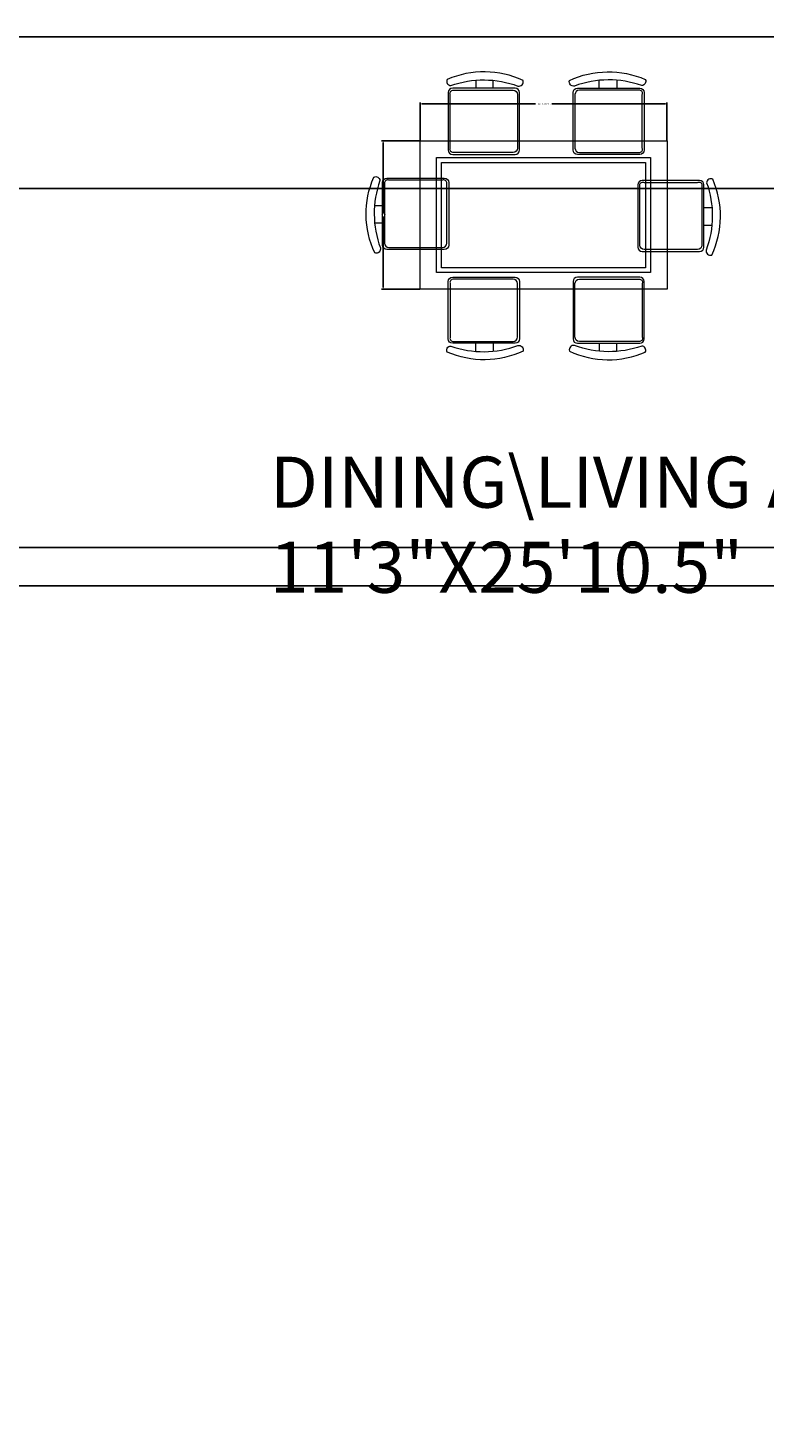
# Model space of a CAD drawing. Units: inches. Extents: x 1355 to 2746, y 1171 to 2751.
# Tile 9 of 24: x 1663 to 1749, y 1818 to 1983. Entities that reach past the tile are written whole.
import ezdxf

# ---------------------------------------------------------------- set-up
doc = ezdxf.new("R2010")
doc.units = ezdxf.units.IN
for name, color, linetype, lineweight in [('A-ANNO-DIMS', 2, 'Continuous', 18), ('A-AREA-IDEN', 7, 'Continuous', 18), ('A-FURN', 8, 'Continuous', 13), ('A-WALL-PATT', 252, 'Continuous', 13)]:
    doc.layers.add(name, color=color, linetype=linetype, lineweight=lineweight)
doc.styles.get("Standard").update_dxf_attribs({"font": 'arial.ttf'})
doc.dimstyles.get("Standard").update_dxf_attribs({"dimtxt": 0.18, "dimasz": 0.18, "dimexe": 0.18, "dimexo": 0.0625, "dimgap": 0.09, "dimtad": 0, "dimtih": 1, "dimtoh": 1, "dimdec": 4, "dimzin": 0, "dimdsep": 46, "dimtxsty": 'Standard', "dimcen": 0.09, "dimadec": 0, "dimazin": 0, "dimtfac": 1, "dimtdec": 4, "dimtofl": 0, "dimtmove": 0, "dimatfit": 3, "dimfxl": 1, "dimtolj": 1, "dimtzin": 0, "dimarcsym": 0})

# ---------------------------------------------------------------- blocks, each defined once
blk = doc.blocks.new('TABLE-DINING')
for points in [[(0, 17.41), (29.01, 17.41), (29.01, 0), (0, 0)], [(1.93, 15.47), (27.08, 15.47), (27.08, 1.93), (1.93, 1.93)], [(2.51, 14.89), (26.5, 14.89), (26.5, 2.51), (2.51, 2.51)]]:
    blk.add_lwpolyline(points, close=True)
blk = doc.blocks.new('*D37')
at = {"layer": 'A-ANNO-DIMS', "color": 0, "lineweight": -2, "transparency": 16777216}
for p, q in [((1708.69, 1969.64), (1708.69, 1974.11)), ((1708.87, 1973.93), (1722.23, 1973.93)), ((1737.52, 1973.93), (1724.16, 1973.93)), ((1737.7, 1969.64), (1737.7, 1974.11))]:
    blk.add_line(p, q, dxfattribs=at)
at = {"layer": 'A-ANNO-DIMS', "color": 0, "transparency": 16777216}
for points in [[(1708.87, 1973.96), (1708.87, 1973.9), (1708.69, 1973.93)], [(1737.52, 1973.96), (1737.52, 1973.9), (1737.7, 1973.93)]]:
    blk.add_solid(points, dxfattribs=at)
at = {"layer": 'Defpoints', "color": 0, "transparency": 16777216}
for p in [(1737.7, 1973.93), (1708.69, 1969.58), (1737.7, 1969.58)]:
    blk.add_point(p, dxfattribs=at)
at = {"layer": 'A-ANNO-DIMS', "color": 0, "transparency": 16777216, "insert": (1723.2, 1973.93), "char_height": 0.18, "attachment_point": 5}
blk.add_mtext('\\A1;TABLE 29 TYP.', dxfattribs=at)
blk = doc.blocks.new('*D38')
at = {"layer": 'A-ANNO-DIMS', "color": 0, "lineweight": -2, "transparency": 16777216}
for p, q in [((1708.63, 1969.58), (1704.16, 1969.58)), ((1704.34, 1969.4), (1704.34, 1961.06)), ((1704.34, 1952.35), (1704.34, 1960.7)), ((1708.63, 1952.17), (1704.16, 1952.17))]:
    blk.add_line(p, q, dxfattribs=at)
at = {"layer": 'A-ANNO-DIMS', "color": 0, "transparency": 16777216}
for points in [[(1704.31, 1969.4), (1704.37, 1969.4), (1704.34, 1969.58)], [(1704.31, 1952.35), (1704.37, 1952.35), (1704.34, 1952.17)]]:
    blk.add_solid(points, dxfattribs=at)
at = {"layer": 'Defpoints', "color": 0, "transparency": 16777216}
for p in [(1704.34, 1969.58), (1708.69, 1969.58), (1708.69, 1952.17)]:
    blk.add_point(p, dxfattribs=at)
at = {"layer": 'A-ANNO-DIMS', "color": 0, "transparency": 16777216, "insert": (1704.34, 1960.88), "char_height": 0.18, "attachment_point": 5}
blk.add_mtext('\\A1;17 TYP.', dxfattribs=at)
blk = doc.blocks.new('*D103')
at = {"layer": 'A-ANNO-DIMS', "color": 0, "lineweight": -2, "transparency": 16777216}
for p, q in [((2089.33, 1917.3), (1407.53, 1917.3)), ((1407.71, 1917.12), (1407.71, 1840.98)), ((1407.71, 1764.48), (1407.71, 1840.62)), ((2089.33, 1764.3), (1407.53, 1764.3))]:
    blk.add_line(p, q, dxfattribs=at)
at = {"layer": 'A-ANNO-DIMS', "color": 0, "transparency": 16777216}
for points in [[(1407.68, 1917.12), (1407.74, 1917.12), (1407.71, 1917.3)], [(1407.68, 1764.48), (1407.74, 1764.48), (1407.71, 1764.3)]]:
    blk.add_solid(points, dxfattribs=at)
at = {"layer": 'Defpoints', "color": 0, "transparency": 16777216}
for p in [(1407.71, 1917.3), (2089.39, 1917.3), (2089.39, 1764.3)]:
    blk.add_point(p, dxfattribs=at)
at = {"layer": 'A-ANNO-DIMS', "color": 0, "transparency": 16777216, "insert": (1407.71, 1840.8), "char_height": 0.18, "attachment_point": 5}
blk.add_mtext('\\A1;153', dxfattribs=at)
blk = doc.blocks.new('*D104')
at = {"layer": 'A-ANNO-DIMS', "color": 0, "lineweight": -2, "transparency": 16777216}
for p, q in [((2089.33, 1986.3), (1407.53, 1986.3)), ((1407.71, 1986.12), (1407.71, 1951.98)), ((1407.71, 1917.48), (1407.71, 1951.62)), ((2089.33, 1917.3), (1407.53, 1917.3))]:
    blk.add_line(p, q, dxfattribs=at)
at = {"layer": 'A-ANNO-DIMS', "color": 0, "transparency": 16777216}
for points in [[(1407.68, 1986.12), (1407.74, 1986.12), (1407.71, 1986.3)], [(1407.68, 1917.48), (1407.74, 1917.48), (1407.71, 1917.3)]]:
    blk.add_solid(points, dxfattribs=at)
at = {"layer": 'Defpoints', "color": 0, "transparency": 16777216}
for p in [(1407.71, 1986.3), (2089.39, 1986.3), (2089.39, 1917.3)]:
    blk.add_point(p, dxfattribs=at)
at = {"layer": 'A-ANNO-DIMS', "color": 0, "transparency": 16777216, "insert": (1407.71, 1951.8), "char_height": 0.18, "attachment_point": 5}
blk.add_mtext('\\A1;69', dxfattribs=at)
blk = doc.blocks.new('*D136')
at = {"layer": 'A-ANNO-DIMS', "color": 0, "lineweight": -2, "transparency": 16777216}
for p, q in [((1618.27, 1981.8), (2648.07, 1981.8)), ((2647.89, 1981.62), (2647.89, 1951.98)), ((2647.89, 1921.98), (2647.89, 1951.62)), ((1618.27, 1921.8), (2648.07, 1921.8))]:
    blk.add_line(p, q, dxfattribs=at)
at = {"layer": 'A-ANNO-DIMS', "color": 0, "transparency": 16777216}
for points in [[(2647.86, 1981.62), (2647.92, 1981.62), (2647.89, 1981.8)], [(2647.86, 1921.98), (2647.92, 1921.98), (2647.89, 1921.8)]]:
    blk.add_solid(points, dxfattribs=at)
at = {"layer": 'Defpoints', "color": 0, "transparency": 16777216}
for p in [(1618.21, 1981.8), (2647.89, 1981.8), (1618.21, 1921.8)]:
    blk.add_point(p, dxfattribs=at)
at = {"layer": 'A-ANNO-DIMS', "color": 0, "transparency": 16777216, "insert": (2647.89, 1951.8), "char_height": 0.18, "attachment_point": 5}
blk.add_mtext('\\A1;60', dxfattribs=at)
blk = doc.blocks.new('*D139')
at = {"layer": 'A-ANNO-DIMS', "color": 0, "lineweight": -2, "transparency": 16777216}
for p, q in [((1523.77, 1981.8), (2648.07, 1981.8)), ((2647.89, 1981.62), (2647.89, 1973.09)), ((2647.89, 1964.19), (2647.89, 1972.72)), ((1548.66, 1964.01), (2648.07, 1964.01))]:
    blk.add_line(p, q, dxfattribs=at)
at = {"layer": 'A-ANNO-DIMS', "color": 0, "transparency": 16777216}
for points in [[(2647.86, 1981.62), (2647.92, 1981.62), (2647.89, 1981.8)], [(2647.86, 1964.19), (2647.92, 1964.19), (2647.89, 1964.01)]]:
    blk.add_solid(points, dxfattribs=at)
at = {"layer": 'Defpoints', "color": 0, "transparency": 16777216}
for p in [(1523.71, 1981.8), (1548.6, 1964.01), (2647.89, 1964.01)]:
    blk.add_point(p, dxfattribs=at)
at = {"layer": 'A-ANNO-DIMS', "color": 0, "transparency": 16777216, "insert": (2647.89, 1972.9), "char_height": 0.18, "attachment_point": 5}
blk.add_mtext('\\A1;17.795', dxfattribs=at)

msp = doc.modelspace()

# ---------------------------------------------------------------- hatches: boundary and pattern name
at = {"layer": 'A-WALL-PATT'}
h = msp.add_hatch(dxfattribs=at)
h.set_pattern_fill('ANSI32', color=256)
h.paths.add_polyline_path([(1660.2083, 2139.3018), (1614.5977, 2139.3018), (1614.5977, 2130.3018), (1655.7083, 2130.3018), (1655.7083, 1981.8018), (1660.2083, 1981.8018), (1660.2083, 2090.7225), (1692.5832, 2090.7225), (1692.5832, 2095.2225), (1660.2083, 2095.2225)])
h.paths.add_polyline_path([(1523.7083, 2130.3018), (1554.5977, 2130.3018), (1554.5977, 2134.8018), (1554.5977, 2139.3018), (1514.7083, 2139.3018), (1514.7083, 2071.8385), (1523.7083, 2071.8385)])
h.paths.add_polyline_path([(1940.7083, 2139.3018), (1883.7928, 2139.3018), (1883.7928, 2130.3018), (1931.7083, 2130.3018), (1931.7083, 2098.3333), (1940.7083, 2098.3333)])
h.paths.add_polyline_path([(1799.7083, 2130.3018), (1823.7928, 2130.3018), (1823.7928, 2134.8018), (1823.7928, 2139.3018), (1795.2083, 2139.3018), (1795.2083, 2130.3018), (1795.2083, 2095.2225), (1759.2134, 2095.2225), (1759.2134, 2090.7225), (1795.2083, 2090.7225), (1795.2083, 1981.8018), (1799.7083, 1981.8018), (1799.7083, 1986.3018)])
h.paths.add_polyline_path([(1940.7083, 2038.3333), (1931.7083, 2038.3333), (1931.7083, 1986.3018), (1832.7083, 1986.3018), (1832.7083, 1947.1338), (1837.2083, 1947.1338), (1837.2083, 1981.8018), (1931.7083, 1981.8018), (1931.7083, 1967.1939), (1940.7083, 1967.1939)])
h.paths.add_polyline_path([(1940.7083, 1943.1939), (1931.7083, 1943.1939), (1931.7083, 1921.8018), (1837.2083, 1921.8018), (1837.2083, 1926.0511), (1832.7083, 1926.0511), (1832.7083, 1917.3018), (1931.7083, 1917.3018), (1931.7083, 1908.3321), (1940.7083, 1908.3321)])
h.paths.add_polyline_path([(1940.7083, 1884.3321), (1931.7083, 1884.3321), (1931.7083, 1869.3018), (1899.4583, 1869.3018), (1899.4583, 1864.8018), (1931.7083, 1864.8018), (1931.7083, 1773.3018), (1786.5143, 1773.3018), (1786.5143, 1764.3018), (1844.7083, 1764.3018), (1844.7083, 1748.9343), (1853.7083, 1748.9343), (1853.7083, 1764.3018), (1931.7083, 1764.3018), (1931.7083, 1652.9424), (1940.7083, 1652.9424)])
h.paths.add_polyline_path([(1799.7083, 1864.8018), (1806.0522, 1864.8018), (1806.0522, 1867.0518), (1806.0522, 1869.3018), (1799.7083, 1869.3018), (1799.7083, 1917.3018), (1799.7083, 1921.8018), (1795.2083, 1921.8018), (1795.2083, 1773.3018), (1799.7083, 1773.3018)])
h.paths.add_polyline_path([(1872.8988, 1867.0518), (1872.8988, 1869.3018), (1867.2083, 1869.3018), (1867.2083, 1917.3018), (1862.7083, 1917.3018), (1862.7083, 1869.3018), (1836.9546, 1869.3018), (1836.9546, 1864.8018), (1862.7083, 1864.8018), (1872.8988, 1864.8018)])
h.paths.add_polyline_path([(1749.2197, 1773.3018), (1655.7083, 1773.3018), (1523.7083, 1773.3018), (1523.7083, 1828.4963), (1514.7083, 1828.4963), (1514.7083, 1753.9033), (1519.2083, 1753.9033), (1523.7083, 1753.9033), (1523.7083, 1764.3018), (1655.7083, 1764.3018), (1749.2197, 1764.3018), (1749.2197, 1768.8018)])
h.paths.add_polyline_path([(1660.2083, 1921.8018), (1655.7083, 1921.8018), (1655.7083, 1917.3018), (1655.7083, 1773.3018), (1660.2083, 1773.3018)])
h.paths.add_polyline_path([(1523.7083, 2011.8385), (1514.7083, 2011.8385), (1514.7083, 1973.114), (1519.2083, 1973.114), (1523.7083, 1973.114), (1523.7083, 1976.8227), (1523.7083, 1981.8018), (1618.2083, 1981.8018), (1618.2083, 1921.8018), (1553.707, 1921.8018), (1553.707, 1917.3018), (1622.7083, 1917.3018), (1622.7083, 1919.5518), (1622.7083, 1921.8018), (1622.7083, 1986.3018), (1523.7083, 1986.3018)])
h.paths.add_polyline_path([(1529.6686, 1919.5518), (1529.6686, 1921.8018), (1523.7083, 1921.8018), (1523.7083, 1949.114), (1514.7083, 1949.114), (1514.7083, 1888.4963), (1523.7083, 1888.4963), (1523.7083, 1917.3018), (1529.6686, 1917.3018)])
h.paths.add_polyline_path([(1538.9419, 1775.643), (1585.5504, 1775.643), (1585.5504, 1798.0318), (1538.9419, 1798.0318)], flags=25)
h.paths.add_polyline_path([(1696.7097, 1497.3356), (1769.5651, 1497.3356), (1769.5651, 1523.4559), (1696.7097, 1523.4559)], flags=9)
h.paths.add_polyline_path([(1629.1643, 1230.5133), (1877.0879, 1230.5133), (1877.0879, 1267.606), (1629.1643, 1267.606)], flags=9)
h.paths.add_polyline_path([(2533.4462, 2215.4033), (2579.9292, 2215.4033), (2579.9292, 2231.889), (2533.4462, 2231.889)], flags=9)
h.paths.add_polyline_path([(2540.822, 2515.6945), (2594.2245, 2515.6945), (2594.2245, 2545.5463), (2540.822, 2545.5463)], flags=9)
h.paths.add_polyline_path([(2535.9857, 2588.2819), (2582.4687, 2588.2819), (2582.4687, 2604.7675), (2535.9857, 2604.7675)], flags=9)
h.paths.add_polyline_path([(2537.1627, 2617.1172), (2649.1245, 2617.1172), (2649.1245, 2633.6029), (2537.1627, 2633.6029)], flags=9)
h.paths.add_polyline_path([(2218.0051, 2168.228), (2363.9573, 2168.228), (2363.9573, 2205.3208), (2218.0051, 2205.3208)], flags=9)
h.paths.add_polyline_path([(1650.2156, 2165.3631), (1800.3547, 2165.3631), (1800.3547, 2202.4559), (1650.2156, 2202.4559)], flags=9)
h.paths.add_polyline_path([(2553.9592, 1610.7663), (2588.4203, 1610.7663), (2588.4203, 1660.2233), (2553.9592, 1660.2233)], flags=9)
h.paths.add_polyline_path([(1549.0868, 1648.2033), (1595.6952, 1648.2033), (1595.6952, 1670.5921), (1549.0868, 1670.5921)], flags=9)
h.paths.add_polyline_path([(1546.9525, 1502.0931), (1583.3413, 1502.0931), (1583.3413, 1524.4819), (1546.9525, 1524.4819)], flags=9)
h.paths.add_polyline_path([(1540.7704, 1433.4431), (1587.3788, 1433.4431), (1587.3788, 1455.8319), (1540.7704, 1455.8319)], flags=9)
h.paths.add_polyline_path([(1683.6524, 1321.5269), (1760.6169, 1321.5269), (1760.6169, 1333.8911), (1683.6524, 1333.8911)], flags=9)
h.paths.add_polyline_path([(1832.0485, 1356.0874), (1873.0989, 1356.0874), (1873.0989, 1378.4762), (1832.0485, 1378.4762)], flags=9)
h.paths.add_polyline_path([(1877.9694, 1431.2138), (1926.3827, 1431.2138), (1926.3827, 1453.578), (1877.9694, 1453.578)], flags=9)
h.paths.add_polyline_path([(1847.3106, 1499.8371), (1883.6994, 1499.8371), (1883.6994, 1522.2259), (1847.3106, 1522.2259)], flags=9)
h.paths.add_polyline_path([(1813.7015, 1640.7287), (1860.3099, 1640.7287), (1860.3099, 1663.1175), (1813.7015, 1663.1175)], flags=9)
h.paths.add_polyline_path([(1876.2576, 1710.2471), (1912.9452, 1710.2471), (1912.9452, 1732.6359), (1876.2576, 1732.6359)], flags=25)
h.paths.add_polyline_path([(1695.9163, 1715.3064), (1736.9668, 1715.3064), (1736.9668, 1737.6952), (1695.9163, 1737.6952)], flags=9)
h.paths.add_polyline_path([(1881.8583, 1888.9094), (1930.2717, 1888.9094), (1930.2717, 1911.2737), (1881.8583, 1911.2737)], flags=9)
h.paths.add_polyline_path([(1823.9298, 1798.6431), (1864.9803, 1798.6431), (1864.9803, 1821.0319), (1823.9298, 1821.0319)], flags=25)
h.paths.add_polyline_path([(1845.6062, 1948.1408), (1881.995, 1948.1408), (1881.995, 1970.5296), (1845.6062, 1970.5296)], flags=25)
h.paths.add_polyline_path([(1849.027, 1991.5151), (1895.6355, 1991.5151), (1895.6355, 2013.9039), (1849.027, 2013.9039)], flags=25)
h.paths.add_polyline_path([(1684.9725, 2113.8416), (1764.2658, 2113.8416), (1764.2658, 2126.2058), (1684.9725, 2126.2058)], flags=9)
h.paths.add_polyline_path([(1688.6193, 1913.0676), (1776.2005, 1913.0676), (1776.2005, 1935.4564), (1688.6193, 1935.4564)], flags=9)
h.paths.add_polyline_path([(1571.4689, 1930.9816), (1607.8577, 1930.9816), (1607.8577, 1953.3704), (1571.4689, 1953.3704)], flags=25)
h.paths.add_polyline_path([(1535.3581, 1998.3125), (1581.9665, 1998.3125), (1581.9665, 2020.7014), (1535.3581, 2020.7014)], flags=9)
h = msp.add_hatch(dxfattribs=at)
h.set_pattern_fill('ANSI32', color=256)
h.paths.add_polyline_path([(1749.2197, 1686.3018), (1732.6892, 1686.3018), (1523.7083, 1686.3018), (1523.7083, 1705.9033), (1514.7083, 1705.9033), (1514.7083, 1647.8732), (1519.2083, 1647.8732), (1523.7083, 1647.8732), (1523.7083, 1677.3018), (1655.7083, 1677.3018), (1655.7083, 1528.8018), (1660.2083, 1528.8018), (1660.2083, 1677.3018), (1732.6892, 1677.3018), (1749.2197, 1677.3018)])
h.paths.add_polyline_path([(1931.7083, 1686.3018), (1853.7083, 1686.3018), (1853.7083, 1703.5696), (1844.7083, 1703.5696), (1844.7083, 1686.3018), (1788.0274, 1686.3018), (1788.0274, 1677.3018), (1795.2083, 1677.3018), (1795.2083, 1528.8018), (1799.7083, 1528.8018), (1799.7083, 1677.3018), (1844.7083, 1677.3018), (1931.7083, 1677.3018)])
h.paths.add_polyline_path([(1931.7083, 1533.3018), (1844.7083, 1533.3018), (1832.7083, 1533.3018), (1832.7083, 1531.0518), (1832.7083, 1528.8018), (1832.7083, 1495.7519), (1837.2083, 1495.7519), (1837.2083, 1528.8018), (1931.7083, 1528.8018)])
h.paths.add_polyline_path([(1940.7083, 1592.9424), (1931.7083, 1592.9424), (1931.7083, 1506.7845), (1940.7083, 1506.7845)])
h.paths.add_polyline_path([(1940.7083, 1482.7845), (1936.2083, 1482.7845), (1931.7083, 1482.7845), (1931.7083, 1320.3018), (1880.7083, 1320.3018), (1880.7083, 1311.3018), (1940.7083, 1311.3018)])
h.paths.add_polyline_path([(1931.7083, 1468.8018), (1844.7083, 1468.8018), (1837.2083, 1468.8018), (1837.2083, 1474.34), (1832.7083, 1474.34), (1832.7083, 1468.8018), (1832.7083, 1464.3018), (1844.7083, 1464.3018), (1931.7083, 1464.3018)])
h.paths.add_polyline_path([(1863.8571, 1464.3018), (1859.3571, 1464.3018), (1859.3571, 1404.1662), (1838.1542, 1404.1662), (1838.1542, 1399.8018), (1869.4185, 1399.8018), (1869.4185, 1402.0518), (1869.4185, 1404.3018), (1863.8571, 1404.3018)])
h.paths.add_polyline_path([(1799.7083, 1399.6662), (1805.4082, 1399.6662), (1805.4082, 1401.9162), (1805.4082, 1404.1662), (1799.7083, 1404.1662), (1799.7083, 1464.3018), (1799.7083, 1468.8018), (1795.2083, 1468.8018), (1795.2083, 1356.2098), (1761.2597, 1356.2098), (1761.2597, 1351.7098), (1795.2083, 1351.7098), (1795.2083, 1320.3018), (1795.2083, 1311.3018), (1844.7083, 1311.3018), (1844.7083, 1315.8018), (1844.7083, 1320.3018), (1799.7083, 1320.3018)])
h.paths.add_polyline_path([(1692.9218, 1356.2098), (1660.2083, 1356.2098), (1660.2083, 1430.786), (1657.9583, 1430.786), (1655.7083, 1430.786), (1655.7083, 1320.3018), (1611.934, 1320.3018), (1611.934, 1311.3018), (1660.2083, 1311.3018), (1660.2083, 1351.7098), (1692.9218, 1351.7098)])
h.paths.add_polyline_path([(1523.7083, 1372.653), (1514.7083, 1372.653), (1514.7083, 1311.3018), (1551.934, 1311.3018), (1551.934, 1315.8018), (1551.934, 1320.3018), (1523.7083, 1320.3018)])
h.paths.add_polyline_path([(1523.7083, 1490.9023), (1514.7083, 1490.9023), (1514.7083, 1432.653), (1519.2083, 1432.653), (1523.7083, 1432.653)])
h.paths.add_polyline_path([(1660.2083, 1468.8018), (1622.7083, 1468.8018), (1622.7083, 1473.1566), (1618.2083, 1473.1566), (1618.2083, 1468.8018), (1523.7083, 1468.8018), (1523.7083, 1464.3018), (1655.7083, 1464.3018), (1655.7083, 1460.5634), (1660.2083, 1460.5634)])
h.paths.add_polyline_path([(1523.7083, 1587.8732), (1514.7083, 1587.8732), (1514.7083, 1514.9023), (1519.2083, 1514.9023), (1523.7083, 1514.9023)])
h.paths.add_polyline_path([(1622.7083, 1533.3018), (1523.7083, 1533.3018), (1523.7083, 1528.8018), (1618.2083, 1528.8018), (1618.2083, 1494.4205), (1622.7083, 1494.4205), (1622.7083, 1528.8018)])
h.paths.add_polyline_path([(1696.7097, 1497.3356), (1769.5651, 1497.3356), (1769.5651, 1523.4559), (1696.7097, 1523.4559)], flags=9)
h.paths.add_polyline_path([(1629.1643, 1230.5133), (1877.0879, 1230.5133), (1877.0879, 1267.606), (1629.1643, 1267.606)], flags=9)
h.paths.add_polyline_path([(2533.4462, 2215.4033), (2579.9292, 2215.4033), (2579.9292, 2231.889), (2533.4462, 2231.889)], flags=9)
h.paths.add_polyline_path([(2540.822, 2515.6945), (2594.2245, 2515.6945), (2594.2245, 2545.5463), (2540.822, 2545.5463)], flags=9)
h.paths.add_polyline_path([(2535.9857, 2588.2819), (2582.4687, 2588.2819), (2582.4687, 2604.7675), (2535.9857, 2604.7675)], flags=9)
h.paths.add_polyline_path([(2537.1627, 2617.1172), (2649.1245, 2617.1172), (2649.1245, 2633.6029), (2537.1627, 2633.6029)], flags=9)
h.paths.add_polyline_path([(2218.0051, 2168.228), (2363.9573, 2168.228), (2363.9573, 2205.3208), (2218.0051, 2205.3208)], flags=9)
h.paths.add_polyline_path([(1650.2156, 2165.3631), (1800.3547, 2165.3631), (1800.3547, 2202.4559), (1650.2156, 2202.4559)], flags=9)
h.paths.add_polyline_path([(2553.9592, 1610.7663), (2588.4203, 1610.7663), (2588.4203, 1660.2233), (2553.9592, 1660.2233)], flags=9)
h.paths.add_polyline_path([(1549.0868, 1648.2033), (1595.6952, 1648.2033), (1595.6952, 1670.5921), (1549.0868, 1670.5921)], flags=25)
h.paths.add_polyline_path([(1546.9525, 1502.0931), (1583.3413, 1502.0931), (1583.3413, 1524.4819), (1546.9525, 1524.4819)], flags=25)
h.paths.add_polyline_path([(1540.7704, 1433.4431), (1587.3788, 1433.4431), (1587.3788, 1455.8319), (1540.7704, 1455.8319)], flags=9)
h.paths.add_polyline_path([(1683.6524, 1321.5269), (1760.6169, 1321.5269), (1760.6169, 1333.8911), (1683.6524, 1333.8911)], flags=9)
h.paths.add_polyline_path([(1832.0485, 1356.0874), (1873.0989, 1356.0874), (1873.0989, 1378.4762), (1832.0485, 1378.4762)], flags=9)
h.paths.add_polyline_path([(1877.9694, 1431.2138), (1926.3827, 1431.2138), (1926.3827, 1453.578), (1877.9694, 1453.578)], flags=9)
h.paths.add_polyline_path([(1847.3106, 1499.8371), (1883.6994, 1499.8371), (1883.6994, 1522.2259), (1847.3106, 1522.2259)], flags=25)
h.paths.add_polyline_path([(1813.7015, 1640.7287), (1860.3099, 1640.7287), (1860.3099, 1663.1175), (1813.7015, 1663.1175)], flags=25)
h.paths.add_polyline_path([(1876.2576, 1710.2471), (1912.9452, 1710.2471), (1912.9452, 1732.6359), (1876.2576, 1732.6359)], flags=9)
h.paths.add_polyline_path([(1695.9163, 1715.3064), (1736.9668, 1715.3064), (1736.9668, 1737.6952), (1695.9163, 1737.6952)], flags=9)
h.paths.add_polyline_path([(1881.8583, 1888.9094), (1930.2717, 1888.9094), (1930.2717, 1911.2737), (1881.8583, 1911.2737)], flags=9)
h.paths.add_polyline_path([(1823.9298, 1798.6431), (1864.9803, 1798.6431), (1864.9803, 1821.0319), (1823.9298, 1821.0319)], flags=9)
h.paths.add_polyline_path([(1845.6062, 1948.1408), (1881.995, 1948.1408), (1881.995, 1970.5296), (1845.6062, 1970.5296)], flags=9)
h.paths.add_polyline_path([(1849.027, 1991.5151), (1895.6355, 1991.5151), (1895.6355, 2013.9039), (1849.027, 2013.9039)], flags=9)
h.paths.add_polyline_path([(1684.9725, 2113.8416), (1764.2658, 2113.8416), (1764.2658, 2126.2058), (1684.9725, 2126.2058)], flags=9)
h.paths.add_polyline_path([(1688.6193, 1913.0676), (1776.2005, 1913.0676), (1776.2005, 1935.4564), (1688.6193, 1935.4564)], flags=9)
h.paths.add_polyline_path([(1538.9419, 1775.643), (1585.5504, 1775.643), (1585.5504, 1798.0318), (1538.9419, 1798.0318)], flags=9)
h.paths.add_polyline_path([(1571.4689, 1930.9816), (1607.8577, 1930.9816), (1607.8577, 1953.3704), (1571.4689, 1953.3704)], flags=9)
h.paths.add_polyline_path([(1535.3581, 1998.3125), (1581.9665, 1998.3125), (1581.9665, 2020.7014), (1535.3581, 2020.7014)], flags=9)

# ---------------------------------------------------------------- linework, layer by layer
at = {"layer": 'A-FURN'}
for points in [[(1712.2794, 1976.0927, -0.17580919), (1720.1811, 1976.0328, 0.57839206), (1720.7797, 1976.691, 0.21452438), (1711.8603, 1976.8107, 0.55201397), (1712.2794, 1976.0927, -0.06507904)], [(1717.2692, 1975.7755), (1717.2692, 1976.7033, -0.06475861)], [(1726.8333, 1976.0328, -0.57839206), (1726.2347, 1976.691, -0.21452438), (1735.154, 1976.8107, -0.55201397), (1734.735, 1976.0927, 0.1758092), (1726.8333, 1976.0328)], [(1729.7452, 1975.7755), (1729.7452, 1976.7033, 0.06475861)], [(1719.8458, 1975.7755), (1712.5102, 1975.7755, 0.41421356), (1711.9969, 1975.2623), (1711.9969, 1968.5173, 0.41421356), (1712.5102, 1968.0041), (1719.8458, 1968.0041, 0.41421356), (1720.359, 1968.5173), (1720.359, 1975.2623, 0.41421356), (1719.8458, 1975.7755)], [(1734.5042, 1975.7755, -0.41421356), (1735.0174, 1975.2623), (1735.0174, 1968.5173, -0.41421356), (1734.5042, 1968.0041), (1727.1685, 1968.0041, -0.41421356), (1726.6553, 1968.5173), (1726.6553, 1975.2623, -0.41421356), (1727.1685, 1975.7755), (1734.5042, 1975.7755)], [(1704.0127, 1957.0112, -0.57839206), (1703.3544, 1956.4126, -0.21452438), (1703.2348, 1965.332, -0.55201397), (1703.9528, 1964.9129, 0.17580937), (1704.0127, 1957.0112)], [(1704.27, 1964.6821, -0.41421356), (1704.7832, 1965.1954), (1711.5282, 1965.1954, -0.41421356), (1712.0414, 1964.6821), (1712.0414, 1957.3465, -0.41421356), (1711.5282, 1956.8333), (1704.7832, 1956.8333, -0.41421356), (1704.27, 1957.3465), (1704.27, 1964.6821)], [(1742.0452, 1964.4309, 0.41421356), (1741.532, 1964.9441), (1734.787, 1964.9441, 0.41421356), (1734.2738, 1964.4309), (1734.2738, 1957.0952, 0.41421356), (1734.787, 1956.582), (1741.532, 1956.582, 0.41421356), (1742.0452, 1957.0952), (1742.0452, 1964.4309)], [(1742.3624, 1964.6617, -0.17580919), (1742.3025, 1956.76, 0.57839206), (1742.9608, 1956.1614, 0.21452438), (1743.0804, 1965.0807, 0.55201397), (1742.3624, 1964.6617, -0.06507904)], [(1704.27, 1959.9231), (1703.3422, 1959.9231, 0.06475861)], [(1742.0452, 1959.6719), (1742.973, 1959.6719, -0.06475861)], [(1719.8458, 1945.7923), (1712.5102, 1945.7923, -0.41421356), (1711.9969, 1946.3055), (1711.9969, 1953.0505, -0.41421356), (1712.5102, 1953.5637), (1719.8458, 1953.5637, -0.41421356), (1720.359, 1953.0505), (1720.359, 1946.3055, -0.41421356), (1719.8458, 1945.7923)], [(1734.5042, 1945.7923, 0.41421356), (1735.0174, 1946.3055), (1735.0174, 1953.0505, 0.41421356), (1734.5042, 1953.5637), (1727.1685, 1953.5637, 0.41421356), (1726.6553, 1953.0505), (1726.6553, 1946.3055, 0.41421356), (1727.1685, 1945.7923), (1734.5042, 1945.7923)], [(1720.1811, 1945.535, -0.57839206), (1720.7797, 1944.8768, -0.21452438), (1711.8603, 1944.7571, -0.55201397), (1712.2794, 1945.4752, 0.17580929), (1720.1811, 1945.535)], [(1717.2692, 1945.7923), (1717.2692, 1944.8646, 0.06475861)], [(1734.735, 1945.4752, -0.17580928), (1726.8333, 1945.535, 0.57839206), (1726.2347, 1944.8768, 0.21452438), (1735.154, 1944.7571, 0.55201397), (1734.735, 1945.4752, -0.06507904)], [(1729.7452, 1945.7923), (1729.7452, 1944.8646, -0.06475861)]]:
    msp.add_lwpolyline(points, format="xyb", dxfattribs=at)
for points in [[(1715.2158, 1976.7201), (1715.2158, 1975.7755)], [(1731.7985, 1976.7201), (1731.7985, 1975.7755)], [(1703.3254, 1961.9765), (1704.27, 1961.9765)], [(1742.9898, 1961.7253), (1742.0452, 1961.7253)], [(1715.2158, 1944.8477), (1715.2158, 1945.7923)], [(1731.7985, 1944.8477), (1731.7985, 1945.7923)]]:
    msp.add_lwpolyline(points, dxfattribs=at)
for points in [[(1712.5133, 1975.5443), (1719.6146, 1975.5443, -0.41421356), (1720.1278, 1975.0311), (1720.1278, 1968.7485, -0.41421356), (1719.6146, 1968.2353), (1712.5133, 1968.2353, -0.51206948), (1712.2281, 1968.7485), (1712.2281, 1975.0311, -0.51206948)], [(1734.5011, 1975.5443), (1727.3997, 1975.5443, 0.41421356), (1726.8865, 1975.0311), (1726.8865, 1968.7485, 0.41421356), (1727.3997, 1968.2353), (1734.5011, 1968.2353, 0.51206948), (1734.7862, 1968.7485), (1734.7862, 1975.0311, 0.51206948)], [(1704.5012, 1964.679), (1704.5012, 1957.5777, 0.41421356), (1705.0144, 1957.0645), (1711.297, 1957.0645, 0.41421356), (1711.8102, 1957.5777), (1711.8102, 1964.679, 0.51206948), (1711.297, 1964.9642), (1705.0144, 1964.9642, 0.51206948)], [(1741.814, 1964.4278), (1741.814, 1957.3265, -0.41421356), (1741.3008, 1956.8132), (1735.0182, 1956.8132, -0.41421356), (1734.505, 1957.3265), (1734.505, 1964.4278, -0.51206948), (1735.0182, 1964.7129), (1741.3008, 1964.7129, -0.51206948)], [(1712.5133, 1946.0235), (1719.6146, 1946.0235, 0.41421356), (1720.1278, 1946.5367), (1720.1278, 1952.8193, 0.41421356), (1719.6146, 1953.3325), (1712.5133, 1953.3325, 0.51206948), (1712.2281, 1952.8193), (1712.2281, 1946.5367, 0.51206948)], [(1734.5011, 1946.0235), (1727.3997, 1946.0235, -0.41421356), (1726.8865, 1946.5367), (1726.8865, 1952.8193, -0.41421356), (1727.3997, 1953.3325), (1734.5011, 1953.3325, -0.51206948), (1734.7862, 1952.8193), (1734.7862, 1946.5367, -0.51206948)]]:
    msp.add_lwpolyline(points, format="xyb", close=True, dxfattribs=at)

# ---------------------------------------------------------------- block references
msp.add_blockref('TABLE-DINING', (1708.691, 1952.174), dxfattribs=at)

# ---------------------------------------------------------------- texts
at = {"layer": 'A-AREA-IDEN', "insert": (1691.032, 1932.4708), "char_height": 6, "attachment_point": 1}
msp.add_mtext_dynamic_manual_height_columns('DINING\\\\LIVING AREA\\P11\'3"X25\'10.5"', width=91.265945, gutter_width=12.5, heights=[0], dxfattribs=at)

# ---------------------------------------------------------------- dimensions: what is measured, and where the dimension line sits
at = {"layer": 'A-ANNO-DIMS'}
for base, p1, p2, override, picture, middle in [((1407.7083, 1986.3018), (2089.3909, 1917.3018), (2089.3909, 1986.3018), {"dimdec": 0, "dimlfac": 1, "dimrnd": 0, "dimzin": 0, "dimdsep": 46, "dimlunit": 2}, '*D104', (1407.7083, 1951.8018)), ((2647.886, 1964.0069), (1523.7083, 1981.8018), (1548.5973, 1964.0069), {"dimdec": 3, "dimlfac": 1, "dimrnd": 0, "dimzin": 0, "dimdsep": 46, "dimlunit": 2}, '*D139', (2647.886, 1972.9044)), ((2647.886, 1981.8018), (1618.2083, 1921.8018), (1618.2083, 1981.8018), {"dimdec": 0, "dimlfac": 1, "dimrnd": 0, "dimzin": 0, "dimdsep": 46, "dimlunit": 2}, '*D136', (2647.886, 1951.8018)), ((1407.7083, 1917.3018), (2089.3909, 1764.3018), (2089.3909, 1917.3018), {"dimdec": 0, "dimlfac": 1, "dimrnd": 0, "dimzin": 0, "dimdsep": 46, "dimlunit": 2}, '*D103', (1407.7083, 1840.8018))]:
    dim = msp.add_linear_dim(base=base, p1=p1, p2=p2, angle=90, dimstyle='Standard', override=override, dxfattribs=at)
    dim.commit()
    dim.dimension.update_dxf_attribs({"geometry": picture, "text_midpoint": middle})
dim = msp.add_linear_dim(base=(1737.7018, 1973.932), p1=(1708.691, 1969.5804), p2=(1737.7018, 1969.5804), text='TABLE <> TYP.', dimstyle='Standard', override={"dimdec": 0, "dimlfac": 1, "dimrnd": 0, "dimzin": 0, "dimdsep": 46, "dimlunit": 2}, dxfattribs=at)
dim.commit()
dim.dimension.update_dxf_attribs({"geometry": '*D37', "text_midpoint": (1723.1964, 1973.932)})
dim = msp.add_linear_dim(base=(1704.3394, 1969.5804), p1=(1708.691, 1952.1739), p2=(1708.691, 1969.5804), angle=90, text='<> TYP.', dimstyle='Standard', override={"dimdec": 0, "dimlfac": 1, "dimrnd": 0, "dimzin": 0, "dimdsep": 46, "dimlunit": 2}, dxfattribs=at)
dim.commit()
dim.dimension.update_dxf_attribs({"geometry": '*D38', "text_midpoint": (1704.3394, 1960.8771)})

doc.saveas('drawing.dxf')
